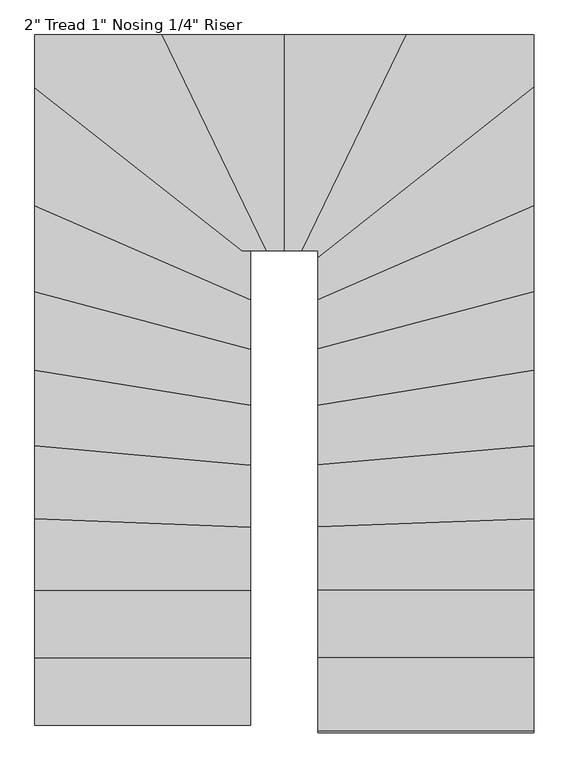
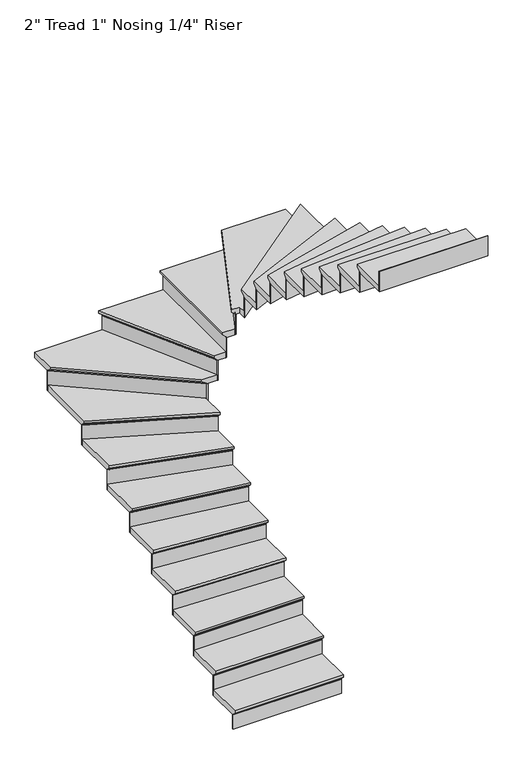
"""IFC4 building model written with IfcOpenShell, lengths in millimetres: stair flight geometry."""

from ifc_helpers import new_model, si_unit, origin, place, context, project, spatial, faceted_brep, source, transform, mapped, element, save


def stair_flight_464fb83d(model_context):
    return source(origin(), model_context, "Body", "Brep", [
        faceted_brep([(-5047.1987704, -4554.2130548, 33073.5214286), (-5047.1987704, -4554.2130548, 33092.5714286), (-5940.8822214, -4554.2130548, 33092.5714286), (-5940.8822214, -4554.2130548, 33073.5214286), (-5047.1987704, -4528.8130548, 33048.1214286), (-5940.8822214, -4528.8130548, 33048.1214286), (-5047.1987704, -4249.4130548, 33092.5714286), (-5940.8822214, -4249.4130548, 33092.5714286), (-5940.8822214, -4528.8130548, 33041.7714286), (-5940.8822214, -4249.4130548, 33041.7714286), (-5047.1987704, -4249.4130548, 33041.7714286), (-5047.1987704, -4528.8130548, 33041.7714286)], [[[0, 1, 2, 3]], [[4, 0, 3, 5]], [[2, 1, 6, 7]], [[8, 9, 10, 11]], [[2, 7, 9, 8, 5, 3]], [[8, 11, 4, 5]], [[6, 1, 0, 4, 11, 10]], [[7, 6, 10, 9]]]),
        faceted_brep([(-5047.1987704, -4528.8130548, 33041.7714286), (-5047.1987704, -4528.8130548, 32918.4), (-5047.1987704, -4522.4630548, 32918.4), (-5047.1987704, -4522.4630548, 33041.7714286), (-5940.8822214, -4528.8130548, 33041.7714286), (-5940.8822214, -4522.4630548, 33041.7714286), (-5940.8822214, -4522.4630548, 32918.4), (-5940.8822214, -4528.8130548, 32918.4)], [[[0, 1, 2, 3]], [[4, 5, 6, 7]], [[1, 0, 4, 7]], [[2, 1, 7, 6]], [[3, 2, 6, 5]], [[0, 3, 5, 4]]]),
        faceted_brep([(-5047.1987704, -4249.4130548, 33215.9428571), (-5047.1987704, -4249.4130548, 33041.7714286), (-5047.1987704, -4243.0630548, 33041.7714286), (-5047.1987704, -4243.0630548, 33215.9428571), (-5940.8822214, -4249.4130548, 33215.9428571), (-5940.8822214, -4243.0630548, 33215.9428571), (-5940.8822214, -4243.0630548, 33041.7714286), (-5940.8822214, -4249.4130548, 33041.7714286)], [[[0, 1, 2, 3]], [[4, 5, 6, 7]], [[1, 0, 4, 7]], [[2, 1, 7, 6]], [[3, 2, 6, 5]], [[0, 3, 5, 4]]]),
        faceted_brep([(-5940.8822214, -4274.8130548, 33266.7428571), (-5047.1987704, -4274.8130548, 33266.7428571), (-5047.1987704, -3970.0130548, 33266.7428571), (-5940.8822214, -3970.0130548, 33266.7428571), (-5940.8822214, -4249.4130548, 33215.9428571), (-5940.8822214, -3970.0130548, 33215.9428571), (-5047.1987704, -3970.0130548, 33215.9428571), (-5047.1987704, -4249.4130548, 33215.9428571), (-5940.8822214, -4249.4130548, 33222.2928571), (-5940.8822214, -4274.8130548, 33247.6928571), (-5047.1987704, -4249.4130548, 33222.2928571), (-5047.1987704, -4274.8130548, 33247.6928571)], [[[0, 1, 2, 3]], [[4, 5, 6, 7]], [[0, 3, 5, 4, 8, 9]], [[4, 7, 10, 8]], [[2, 1, 11, 10, 7, 6]], [[3, 2, 6, 5]], [[11, 1, 0, 9]], [[10, 11, 9, 8]]]),
        faceted_brep([(-5047.1987704, -3970.0130548, 33390.1142857), (-5047.1987704, -3970.0130548, 33215.9428571), (-5047.1987704, -3963.6630548, 33215.9428571), (-5047.1987704, -3963.6630548, 33390.1142857), (-5940.8822214, -3970.0130548, 33390.1142857), (-5940.8822214, -3963.6630548, 33390.1142857), (-5940.8822214, -3963.6630548, 33215.9428571), (-5940.8822214, -3970.0130548, 33215.9428571)], [[[0, 1, 2, 3]], [[4, 5, 6, 7]], [[1, 0, 4, 7]], [[2, 1, 7, 6]], [[3, 2, 6, 5]], [[0, 3, 5, 4]]]),
        faceted_brep([(-5940.8822214, -3995.4130548, 33440.9142857), (-5047.1987704, -3995.4130548, 33440.9142857), (-5047.1987704, -3707.9036879, 33440.9142857), (-5940.8822214, -3673.2843203, 33440.9142857), (-5940.8822214, -3970.0130548, 33390.1142857), (-5940.8822214, -3673.2843203, 33390.1142857), (-5047.1987704, -3707.9036879, 33390.1142857), (-5047.1987704, -3970.0130548, 33390.1142857), (-5940.8822214, -3970.0130548, 33396.4642857), (-5940.8822214, -3995.4130548, 33421.8642857), (-5047.1987704, -3970.0130548, 33396.4642857), (-5047.1987704, -3995.4130548, 33421.8642857)], [[[0, 1, 2, 3]], [[4, 5, 6, 7]], [[0, 3, 5, 4, 8, 9]], [[4, 7, 10, 8]], [[2, 1, 11, 10, 7, 6]], [[3, 2, 6, 5]], [[11, 1, 0, 9]], [[10, 11, 9, 8]]]),
        faceted_brep([(-5047.1987704, -3707.9036879, 33564.2857143), (-5047.1987704, -3707.9036879, 33390.1142857), (-5047.1987704, -3701.5489252, 33390.1142857), (-5047.1987704, -3701.5489252, 33564.2857143), (-5940.8822214, -3673.2843203, 33564.2857143), (-5940.8822214, -3666.9295576, 33564.2857143), (-5940.8822214, -3666.9295576, 33390.1142857), (-5940.8822214, -3673.2843203, 33390.1142857)], [[[0, 1, 2, 3]], [[4, 5, 6, 7]], [[1, 0, 4, 7]], [[2, 1, 7, 6]], [[3, 2, 6, 5]], [[0, 3, 5, 4]]]),
        faceted_brep([(-5940.8822214, -3698.703371, 33615.0857143), (-5047.1987704, -3733.3227386, 33615.0857143), (-5047.1987704, -3451.3234819, 33615.0857143), (-5940.8822214, -3370.89733, 33615.0857143), (-5940.8822214, -3673.2843203, 33564.2857143), (-5940.8822214, -3370.89733, 33564.2857143), (-5047.1987704, -3451.3234819, 33564.2857143), (-5047.1987704, -3707.9036879, 33564.2857143), (-5940.8822214, -3673.2843203, 33570.6357143), (-5940.8822214, -3698.703371, 33596.0357143), (-5047.1987704, -3707.9036879, 33570.6357143), (-5047.1987704, -3733.3227386, 33596.0357143)], [[[0, 1, 2, 3]], [[4, 5, 6, 7]], [[0, 3, 5, 4, 8, 9]], [[4, 7, 10, 8]], [[2, 1, 11, 10, 7, 6]], [[3, 2, 6, 5]], [[11, 1, 0, 9]], [[10, 11, 9, 8]]]),
        faceted_brep([(-5047.1987704, -3451.3234819, 33738.4571429), (-5047.1987704, -3451.3234819, 33564.2857143), (-5047.1987704, -3444.9478197, 33564.2857143), (-5047.1987704, -3444.9478197, 33738.4571429), (-5940.8822214, -3370.89733, 33738.4571429), (-5940.8822214, -3364.5216678, 33738.4571429), (-5940.8822214, -3364.5216678, 33564.2857143), (-5940.8822214, -3370.89733, 33564.2857143)], [[[0, 1, 2, 3]], [[4, 5, 6, 7]], [[1, 0, 4, 7]], [[2, 1, 7, 6]], [[3, 2, 6, 5]], [[0, 3, 5, 4]]]),
        faceted_brep([(-5940.8822214, -3396.3999789, 33789.2571429), (-5047.1987704, -3476.8261308, 33789.2571429), (-5047.1987704, -3203.4301079, 33789.2571429), (-5940.8822214, -3059.5417727, 33789.2571429), (-5940.8822214, -3370.89733, 33738.4571429), (-5940.8822214, -3059.5417727, 33738.4571429), (-5047.1987704, -3203.4301079, 33738.4571429), (-5047.1987704, -3451.3234819, 33738.4571429), (-5940.8822214, -3370.89733, 33744.8071429), (-5940.8822214, -3396.3999789, 33770.2071429), (-5047.1987704, -3451.3234819, 33744.8071429), (-5047.1987704, -3476.8261308, 33770.2071429)], [[[0, 1, 2, 3]], [[4, 5, 6, 7]], [[0, 3, 5, 4, 8, 9]], [[4, 7, 10, 8]], [[2, 1, 11, 10, 7, 6]], [[3, 2, 6, 5]], [[11, 1, 0, 9]], [[10, 11, 9, 8]]]),
        faceted_brep([(-5047.1987704, -3203.4301079, 33912.6285714), (-5047.1987704, -3203.4301079, 33738.4571429), (-5047.1987704, -3196.9983292, 33738.4571429), (-5047.1987704, -3196.9983292, 33912.6285714), (-5940.8822214, -3059.5417727, 33912.6285714), (-5940.8822214, -3053.109994, 33912.6285714), (-5940.8822214, -3053.109994, 33738.4571429), (-5940.8822214, -3059.5417727, 33738.4571429)], [[[0, 1, 2, 3]], [[4, 5, 6, 7]], [[1, 0, 4, 7]], [[2, 1, 7, 6]], [[3, 2, 6, 5]], [[0, 3, 5, 4]]]),
        faceted_brep([(-5940.8822214, -3085.2688872, 33963.4285714), (-5047.1987704, -3229.1572224, 33963.4285714), (-5047.1987704, -2970.3553609, 33963.4285714), (-5940.8822214, -2732.7052783, 33963.4285714), (-5940.8822214, -3059.5417727, 33912.6285714), (-5940.8822214, -2732.7052783, 33912.6285714), (-5047.1987704, -2970.3553609, 33912.6285714), (-5047.1987704, -3203.4301079, 33912.6285714), (-5940.8822214, -3059.5417727, 33918.9785714), (-5940.8822214, -3085.2688872, 33944.3785714), (-5047.1987704, -3203.4301079, 33918.9785714), (-5047.1987704, -3229.1572224, 33944.3785714)], [[[0, 1, 2, 3]], [[4, 5, 6, 7]], [[0, 3, 5, 4, 8, 9]], [[4, 7, 10, 8]], [[2, 1, 11, 10, 7, 6]], [[3, 2, 6, 5]], [[11, 1, 0, 9]], [[10, 11, 9, 8]]]),
        faceted_brep([(-5047.1987704, -2970.3553609, 34086.8), (-5047.1987704, -2970.3553609, 33912.6285714), (-5047.1987704, -2963.7846771, 33912.6285714), (-5047.1987704, -2963.7846771, 34086.8), (-5940.8822214, -2732.7052783, 34086.8), (-5940.8822214, -2726.1345945, 34086.8), (-5940.8822214, -2726.1345945, 33912.6285714), (-5940.8822214, -2732.7052783, 33912.6285714)], [[[0, 1, 2, 3]], [[4, 5, 6, 7]], [[1, 0, 4, 7]], [[2, 1, 7, 6]], [[3, 2, 6, 5]], [[0, 3, 5, 4]]]),
        faceted_brep([(-5940.8822214, -2758.9880136, 34137.6), (-5047.1987704, -2996.6380961, 34137.6), (-5047.1987704, -2765.8050203, 34137.6), (-5940.8822214, -2375.5896532, 34137.6), (-5940.8822214, -2732.7052783, 34086.8), (-5940.8822214, -2375.5896532, 34086.8), (-5047.1987704, -2765.8050203, 34086.8), (-5047.1987704, -2970.3553609, 34086.8), (-5940.8822214, -2732.7052783, 34093.15), (-5940.8822214, -2758.9880136, 34118.55), (-5047.1987704, -2970.3553609, 34093.15), (-5047.1987704, -2996.6380961, 34118.55)], [[[0, 1, 2, 3]], [[4, 5, 6, 7]], [[0, 3, 5, 4, 8, 9]], [[4, 7, 10, 8]], [[2, 1, 11, 10, 7, 6]], [[3, 2, 6, 5]], [[11, 1, 0, 9]], [[10, 11, 9, 8]]]),
        faceted_brep([(-5047.1987704, -2765.8050203, 34260.9714286), (-5047.1987704, -2765.8050203, 34086.8), (-5047.1987704, -2758.8760908, 34086.8), (-5047.1987704, -2758.8760908, 34260.9714286), (-5940.8822214, -2375.5896532, 34260.9714286), (-5940.8822214, -2368.6607237, 34260.9714286), (-5940.8822214, -2368.6607237, 34086.8), (-5940.8822214, -2375.5896532, 34086.8)], [[[0, 1, 2, 3]], [[4, 5, 6, 7]], [[1, 0, 4, 7]], [[2, 1, 7, 6]], [[3, 2, 6, 5]], [[0, 3, 5, 4]]]),
        faceted_brep([(-5940.8822214, -2403.3053713, 34311.7714286), (-5047.1987704, -2793.5207384, 34311.7714286), (-5047.1987704, -2590.8424524, 34311.7714286), (-5040.8038639, -2590.8424524, 34311.7714286), (-5940.8822214, -1882.1944717, 34311.7714286), (-5940.8822214, -2375.5896532, 34260.9714286), (-5940.8822214, -1882.1944717, 34260.9714286), (-5040.8038639, -2590.8424524, 34260.9714286), (-5047.1987704, -2590.8424524, 34260.9714286), (-5047.1987704, -2765.8050203, 34260.9714286), (-5940.8822214, -2375.5896532, 34267.3214286), (-5940.8822214, -2403.3053713, 34292.7214286), (-5047.1987704, -2765.8050203, 34267.3214286), (-5047.1987704, -2793.5207384, 34292.7214286)], [[[0, 1, 2, 3, 4]], [[5, 6, 7, 8, 9]], [[0, 4, 6, 5, 10, 11]], [[5, 9, 12, 10]], [[2, 1, 13, 12, 9, 8]], [[4, 3, 7, 6]], [[13, 1, 0, 11]], [[12, 13, 11, 10]], [[3, 2, 8, 7]]]),
        faceted_brep([(-5040.8038639, -2590.8424524, 34435.1428571), (-5040.8038639, -2590.8424524, 34260.9714286), (-5030.5387554, -2590.8424524, 34260.9714286), (-5030.5387554, -2590.8424524, 34435.1428571), (-5940.8822214, -1882.1944717, 34435.1428571), (-5940.8822214, -1874.1125661, 34435.1428571), (-5940.8822214, -1874.1125661, 34260.9714286), (-5940.8822214, -1882.1944717, 34260.9714286)], [[[0, 1, 2, 3]], [[4, 5, 6, 7]], [[1, 0, 4, 7]], [[2, 1, 7, 6]], [[3, 2, 6, 5]], [[0, 3, 5, 4]]]),
        faceted_brep([(-5384.6489457, -1697.1590014, 34485.9428571), (-5940.8822214, -1697.1590014, 34485.9428571), (-5940.8822214, -1914.5220945, 34485.9428571), (-5081.8642978, -2590.8424524, 34485.9428571), (-4952.3566185, -2590.8424524, 34485.9428571), (-5940.8822214, -1697.1590014, 34435.1428571), (-5384.6489457, -1697.1590014, 34435.1428571), (-4952.3566185, -2590.8424524, 34435.1428571), (-5040.8038639, -2590.8424524, 34435.1428571), (-5940.8822214, -1882.1944717, 34435.1428571), (-5940.8822214, -1882.1944717, 34441.4928571), (-5940.8822214, -1914.5220945, 34466.8928571), (-5040.8038639, -2590.8424524, 34441.4928571), (-5081.8642978, -2590.8424524, 34466.8928571)], [[[0, 1, 2, 3, 4]], [[5, 6, 7, 8, 9]], [[1, 0, 6, 5]], [[2, 1, 5, 9, 10, 11]], [[9, 8, 12, 10]], [[4, 3, 13, 12, 8, 7]], [[0, 4, 7, 6]], [[13, 3, 2, 11]], [[12, 13, 11, 10]]]),
        faceted_brep([(-4952.3566185, -2590.8424524, 34609.3142857), (-4952.3566185, -2590.8424524, 34435.1428571), (-4945.3027294, -2590.8424524, 34435.1428571), (-4945.3027294, -2590.8424524, 34609.3142857), (-5384.6489457, -1697.1590014, 34609.3142857), (-5377.5950566, -1697.1590014, 34609.3142857), (-5377.5950566, -1697.1590014, 34435.1428571), (-5384.6489457, -1697.1590014, 34435.1428571)], [[[0, 1, 2, 3]], [[4, 5, 6, 7]], [[1, 0, 4, 7]], [[2, 1, 7, 6]], [[3, 2, 6, 5]], [[0, 3, 5, 4]]]),
        faceted_brep([(-5412.8645022, -1697.1590014, 34660.1142857), (-4980.5721749, -2590.8424524, 34660.1142857), (-4882.0987704, -2590.8424524, 34660.1142857), (-4882.0987706, -1697.1590014, 34660.1142857), (-5384.6489457, -1697.1590014, 34609.3142857), (-4882.0987706, -1697.1590014, 34609.3142857), (-4882.0987704, -2590.8424524, 34609.3142857), (-4952.3566185, -2590.8424524, 34609.3142857), (-5384.6489457, -1697.1590014, 34615.6642857), (-5412.8645022, -1697.1590014, 34641.0642857), (-4952.3566185, -2590.8424524, 34615.6642857), (-4980.5721749, -2590.8424524, 34641.0642857)], [[[0, 1, 2, 3]], [[4, 5, 6, 7]], [[0, 3, 5, 4, 8, 9]], [[4, 7, 10, 8]], [[3, 2, 6, 5]], [[11, 1, 0, 9]], [[10, 11, 9, 8]], [[2, 1, 11, 10, 7, 6]]]),
        faceted_brep([(-4882.0987704, -2590.8424524, 34783.4857143), (-4882.0987704, -2590.8424524, 34609.3142857), (-4875.7487704, -2590.8424524, 34609.3142857), (-4875.7487704, -2590.8424524, 34783.4857143), (-4882.0987706, -1697.1590014, 34783.4857143), (-4875.7487706, -1697.1590014, 34783.4857143), (-4875.7487706, -1697.1590014, 34609.3142857), (-4882.0987706, -1697.1590014, 34609.3142857)], [[[0, 1, 2, 3]], [[4, 5, 6, 7]], [[1, 0, 4, 7]], [[2, 1, 7, 6]], [[3, 2, 6, 5]], [[0, 3, 5, 4]]]),
        faceted_brep([(-4907.4987706, -1697.1590014, 34834.2857143), (-4907.4987704, -2590.8424524, 34834.2857143), (-4806.2098095, -2590.8424524, 34834.2857143), (-4373.9174828, -1697.1590014, 34834.2857143), (-4882.0987706, -1697.1590014, 34783.4857143), (-4373.9174828, -1697.1590014, 34783.4857143), (-4806.2098095, -2590.8424524, 34783.4857143), (-4882.0987704, -2590.8424524, 34783.4857143), (-4882.0987706, -1697.1590014, 34789.8357143), (-4907.4987706, -1697.1590014, 34815.2357143), (-4882.0987704, -2590.8424524, 34789.8357143), (-4907.4987704, -2590.8424524, 34815.2357143)], [[[0, 1, 2, 3]], [[4, 5, 6, 7]], [[0, 3, 5, 4, 8, 9]], [[4, 7, 10, 8]], [[2, 1, 11, 10, 7, 6]], [[3, 2, 6, 5]], [[11, 1, 0, 9]], [[10, 11, 9, 8]]]),
        faceted_brep([(-4806.2098095, -2590.8424524, 34957.6571429), (-4806.2098095, -2590.8424524, 34783.4857143), (-4799.1559204, -2590.8424524, 34783.4857143), (-4799.1559204, -2590.8424524, 34957.6571429), (-4373.9174828, -1697.1590014, 34957.6571429), (-4366.8635937, -1697.1590014, 34957.6571429), (-4366.8635937, -1697.1590014, 34783.4857143), (-4373.9174828, -1697.1590014, 34783.4857143)], [[[0, 1, 2, 3]], [[4, 5, 6, 7]], [[1, 0, 4, 7]], [[2, 1, 7, 6]], [[3, 2, 6, 5]], [[0, 3, 5, 4]]]),
        faceted_brep([(-3874.1153195, -1946.8497166, 35008.4571429), (-3874.1153195, -1697.1590014, 35008.4571429), (-4402.1330392, -1697.1590014, 35008.4571429), (-4834.4253659, -2590.8424524, 35008.4571429), (-4767.7987704, -2590.8424524, 35008.4571429), (-4767.7987704, -2650.4628721, 35008.4571429), (-3874.1153195, -1697.1590014, 34957.6571429), (-3874.1153195, -1946.8497166, 34957.6571429), (-4767.7987704, -2650.4628721, 34957.6571429), (-4767.7987704, -2590.8424524, 34957.6571429), (-4806.2098095, -2590.8424524, 34957.6571429), (-4373.9174828, -1697.1590014, 34957.6571429), (-4806.2098095, -2590.8424524, 34964.0071429), (-4373.9174828, -1697.1590014, 34964.0071429), (-4834.4253659, -2590.8424524, 34989.4071429), (-4402.1330392, -1697.1590014, 34989.4071429)], [[[0, 1, 2, 3, 4, 5]], [[6, 7, 8, 9, 10, 11]], [[1, 0, 7, 6]], [[11, 10, 12, 13]], [[4, 3, 14, 12, 10, 9]], [[5, 4, 9, 8]], [[0, 5, 8, 7]], [[14, 3, 2, 15]], [[12, 14, 15, 13]], [[2, 1, 6, 11, 13, 15]]]),
        faceted_brep([(-4767.7987704, -2650.4628721, 35131.8285714), (-4767.7987704, -2650.4628721, 34957.6571429), (-4767.7987704, -2658.5447778, 34957.6571429), (-4767.7987704, -2658.5447778, 35131.8285714), (-3874.1153195, -1946.8497166, 35131.8285714), (-3874.1153195, -1954.9316222, 35131.8285714), (-3874.1153195, -1954.9316222, 34957.6571429), (-3874.1153195, -1946.8497166, 34957.6571429)], [[[0, 1, 2, 3]], [[4, 5, 6, 7]], [[1, 0, 4, 7]], [[2, 1, 7, 6]], [[3, 2, 6, 5]], [[0, 3, 5, 4]]]),
        faceted_brep([(-3874.1153195, -1914.5220938, 35182.6285714), (-4767.7987704, -2618.1352494, 35182.6285714), (-4767.7987704, -2821.2364563, 35182.6285714), (-3874.1153195, -2431.0210889, 35182.6285714), (-3874.1153195, -1946.8497166, 35131.8285714), (-3874.1153195, -2431.0210889, 35131.8285714), (-4767.7987704, -2821.2364563, 35131.8285714), (-4767.7987704, -2650.4628721, 35131.8285714), (-3874.1153195, -1946.8497166, 35138.1785714), (-3874.1153195, -1914.5220938, 35163.5785714), (-4767.7987704, -2650.4628721, 35138.1785714), (-4767.7987704, -2618.1352494, 35163.5785714)], [[[0, 1, 2, 3]], [[4, 5, 6, 7]], [[0, 3, 5, 4, 8, 9]], [[4, 7, 10, 8]], [[2, 1, 11, 10, 7, 6]], [[3, 2, 6, 5]], [[11, 1, 0, 9]], [[10, 11, 9, 8]]]),
        faceted_brep([(-4767.7987704, -2821.2364563, 35306.0), (-4767.7987704, -2821.2364563, 35131.8285714), (-4767.7987704, -2828.1653858, 35131.8285714), (-4767.7987704, -2828.1653858, 35306.0), (-3874.1153195, -2431.0210889, 35306.0), (-3874.1153195, -2437.9500185, 35306.0), (-3874.1153195, -2437.9500185, 35131.8285714), (-3874.1153195, -2431.0210889, 35131.8285714)], [[[0, 1, 2, 3]], [[4, 5, 6, 7]], [[1, 0, 4, 7]], [[2, 1, 7, 6]], [[3, 2, 6, 5]], [[0, 3, 5, 4]]]),
        faceted_brep([(-3874.1153195, -2403.3053709, 35356.8), (-4767.7987704, -2793.5207382, 35356.8), (-4767.7987704, -3022.9208311, 35356.8), (-3874.1153195, -2785.2707484, 35356.8), (-3874.1153195, -2431.0210889, 35306.0), (-3874.1153195, -2785.2707484, 35306.0), (-4767.7987704, -3022.9208311, 35306.0), (-4767.7987704, -2821.2364563, 35306.0), (-3874.1153195, -2431.0210889, 35312.35), (-3874.1153195, -2403.3053709, 35337.75), (-4767.7987704, -2821.2364563, 35312.35), (-4767.7987704, -2793.5207382, 35337.75)], [[[0, 1, 2, 3]], [[4, 5, 6, 7]], [[0, 3, 5, 4, 8, 9]], [[4, 7, 10, 8]], [[2, 1, 11, 10, 7, 6]], [[3, 2, 6, 5]], [[11, 1, 0, 9]], [[10, 11, 9, 8]]]),
        faceted_brep([(-4767.7987704, -3022.9208311, 35480.1714286), (-4767.7987704, -3022.9208311, 35306.0), (-4767.7987704, -3029.4915149, 35306.0), (-4767.7987704, -3029.4915149, 35480.1714286), (-3874.1153195, -2785.2707484, 35480.1714286), (-3874.1153195, -2791.8414322, 35480.1714286), (-3874.1153195, -2791.8414322, 35306.0), (-3874.1153195, -2785.2707484, 35306.0)], [[[0, 1, 2, 3]], [[4, 5, 6, 7]], [[1, 0, 4, 7]], [[2, 1, 7, 6]], [[3, 2, 6, 5]], [[0, 3, 5, 4]]]),
        faceted_brep([(-3874.1153195, -2758.9880132, 35530.9714286), (-4767.7987704, -2996.6380959, 35530.9714286), (-4767.7987704, -3254.8843368, 35530.9714286), (-3874.1153195, -3110.9960015, 35530.9714286), (-3874.1153195, -2785.2707484, 35480.1714286), (-3874.1153195, -3110.9960015, 35480.1714286), (-4767.7987704, -3254.8843368, 35480.1714286), (-4767.7987704, -3022.9208311, 35480.1714286), (-3874.1153195, -2785.2707484, 35486.5214286), (-3874.1153195, -2758.9880132, 35511.9214286), (-4767.7987704, -3022.9208311, 35486.5214286), (-4767.7987704, -2996.6380959, 35511.9214286)], [[[0, 1, 2, 3]], [[4, 5, 6, 7]], [[0, 3, 5, 4, 8, 9]], [[4, 7, 10, 8]], [[2, 1, 11, 10, 7, 6]], [[3, 2, 6, 5]], [[11, 1, 0, 9]], [[10, 11, 9, 8]]]),
        faceted_brep([(-4767.7987704, -3254.8843368, 35654.3428571), (-4767.7987704, -3254.8843368, 35480.1714286), (-4767.7987704, -3261.3161154, 35480.1714286), (-4767.7987704, -3261.3161154, 35654.3428571), (-3874.1153195, -3110.9960015, 35654.3428571), (-3874.1153195, -3117.4277801, 35654.3428571), (-3874.1153195, -3117.4277801, 35480.1714286), (-3874.1153195, -3110.9960015, 35480.1714286)], [[[0, 1, 2, 3]], [[4, 5, 6, 7]], [[1, 0, 4, 7]], [[2, 1, 7, 6]], [[3, 2, 6, 5]], [[0, 3, 5, 4]]]),
        faceted_brep([(-3874.1153195, -3085.2688869, 35705.1428571), (-4767.7987704, -3229.1572222, 35705.1428571), (-4767.7987704, -3502.3287795, 35705.1428571), (-3874.1153195, -3421.9026274, 35705.1428571), (-3874.1153195, -3110.9960015, 35654.3428571), (-3874.1153195, -3421.9026274, 35654.3428571), (-4767.7987704, -3502.3287795, 35654.3428571), (-4767.7987704, -3254.8843368, 35654.3428571), (-3874.1153195, -3110.9960015, 35660.6928571), (-3874.1153195, -3085.2688869, 35686.0928571), (-4767.7987704, -3254.8843368, 35660.6928571), (-4767.7987704, -3229.1572222, 35686.0928571)], [[[0, 1, 2, 3]], [[4, 5, 6, 7]], [[0, 3, 5, 4, 8, 9]], [[4, 7, 10, 8]], [[2, 1, 11, 10, 7, 6]], [[3, 2, 6, 5]], [[11, 1, 0, 9]], [[10, 11, 9, 8]]]),
        faceted_brep([(-4767.7987704, -3502.3287795, 35828.5142857), (-4767.7987704, -3502.3287795, 35654.3428571), (-4767.7987704, -3508.7044417, 35654.3428571), (-4767.7987704, -3508.7044417, 35828.5142857), (-3874.1153195, -3421.9026274, 35828.5142857), (-3874.1153195, -3428.2782897, 35828.5142857), (-3874.1153195, -3428.2782897, 35654.3428571), (-3874.1153195, -3421.9026274, 35654.3428571)], [[[0, 1, 2, 3]], [[4, 5, 6, 7]], [[1, 0, 4, 7]], [[2, 1, 7, 6]], [[3, 2, 6, 5]], [[0, 3, 5, 4]]]),
        faceted_brep([(-3874.1153195, -3396.3999786, 35879.3142857), (-4767.7987704, -3476.8261306, 35879.3142857), (-4767.7987704, -3758.7417891, 35879.3142857), (-3874.1153195, -3724.1224215, 35879.3142857), (-3874.1153195, -3421.9026274, 35828.5142857), (-3874.1153195, -3724.1224215, 35828.5142857), (-4767.7987704, -3758.7417891, 35828.5142857), (-4767.7987704, -3502.3287795, 35828.5142857), (-3874.1153195, -3421.9026274, 35834.8642857), (-3874.1153195, -3396.3999786, 35860.2642857), (-4767.7987704, -3502.3287795, 35834.8642857), (-4767.7987704, -3476.8261306, 35860.2642857)], [[[0, 1, 2, 3]], [[4, 5, 6, 7]], [[0, 3, 5, 4, 8, 9]], [[4, 7, 10, 8]], [[2, 1, 11, 10, 7, 6]], [[3, 2, 6, 5]], [[11, 1, 0, 9]], [[10, 11, 9, 8]]]),
        faceted_brep([(-4767.7987704, -3758.7417891, 36002.6857143), (-4767.7987704, -3758.7417891, 35828.5142857), (-4767.7987704, -3765.0965518, 35828.5142857), (-4767.7987704, -3765.0965518, 36002.6857143), (-3874.1153195, -3724.1224215, 36002.6857143), (-3874.1153195, -3730.4771842, 36002.6857143), (-3874.1153195, -3730.4771842, 35828.5142857), (-3874.1153195, -3724.1224215, 35828.5142857)], [[[0, 1, 2, 3]], [[4, 5, 6, 7]], [[1, 0, 4, 7]], [[2, 1, 7, 6]], [[3, 2, 6, 5]], [[0, 3, 5, 4]]]),
        faceted_brep([(-3874.1153195, -3698.7033708, 36053.4857143), (-4767.7987704, -3733.3227384, 36053.4857143), (-4767.7987704, -4020.8130546, 36053.4857143), (-3874.1153195, -4020.8130546, 36053.4857143), (-3874.1153195, -3724.1224215, 36002.6857143), (-3874.1153195, -4020.8130546, 36002.6857143), (-4767.7987704, -4020.8130546, 36002.6857143), (-4767.7987704, -3758.7417891, 36002.6857143), (-3874.1153195, -3724.1224215, 36009.0357143), (-3874.1153195, -3698.7033708, 36034.4357143), (-4767.7987704, -3758.7417891, 36009.0357143), (-4767.7987704, -3733.3227384, 36034.4357143)], [[[0, 1, 2, 3]], [[4, 5, 6, 7]], [[0, 3, 5, 4, 8, 9]], [[4, 7, 10, 8]], [[2, 1, 11, 10, 7, 6]], [[3, 2, 6, 5]], [[11, 1, 0, 9]], [[10, 11, 9, 8]]]),
        faceted_brep([(-4767.7987704, -4020.8130546, 36176.8571429), (-4767.7987704, -4020.8130546, 36002.6857143), (-4767.7987704, -4027.1630546, 36002.6857143), (-4767.7987704, -4027.1630546, 36176.8571429), (-3874.1153195, -4020.8130546, 36176.8571429), (-3874.1153195, -4027.1630546, 36176.8571429), (-3874.1153195, -4027.1630546, 36002.6857143), (-3874.1153195, -4020.8130546, 36002.6857143)], [[[0, 1, 2, 3]], [[4, 5, 6, 7]], [[1, 0, 4, 7]], [[2, 1, 7, 6]], [[3, 2, 6, 5]], [[0, 3, 5, 4]]]),
        faceted_brep([(-3874.1153195, -3995.4130546, 36227.6571429), (-4767.7987704, -3995.4130546, 36227.6571429), (-4767.7987704, -4300.2130546, 36227.6571429), (-3874.1153195, -4300.2130546, 36227.6571429), (-3874.1153195, -4020.8130546, 36176.8571429), (-3874.1153195, -4300.2130546, 36176.8571429), (-4767.7987704, -4300.2130546, 36176.8571429), (-4767.7987704, -4020.8130546, 36176.8571429), (-3874.1153195, -4020.8130546, 36183.2071429), (-3874.1153195, -3995.4130546, 36208.6071429), (-4767.7987704, -4020.8130546, 36183.2071429), (-4767.7987704, -3995.4130546, 36208.6071429)], [[[0, 1, 2, 3]], [[4, 5, 6, 7]], [[0, 3, 5, 4, 8, 9]], [[4, 7, 10, 8]], [[2, 1, 11, 10, 7, 6]], [[3, 2, 6, 5]], [[11, 1, 0, 9]], [[10, 11, 9, 8]]]),
        faceted_brep([(-4767.7987704, -4300.2130546, 36351.0285714), (-4767.7987704, -4300.2130546, 36176.8571429), (-4767.7987704, -4306.5630546, 36176.8571429), (-4767.7987704, -4306.5630546, 36351.0285714), (-3874.1153195, -4300.2130546, 36351.0285714), (-3874.1153195, -4306.5630546, 36351.0285714), (-3874.1153195, -4306.5630546, 36176.8571429), (-3874.1153195, -4300.2130546, 36176.8571429)], [[[0, 1, 2, 3]], [[4, 5, 6, 7]], [[1, 0, 4, 7]], [[2, 1, 7, 6]], [[3, 2, 6, 5]], [[0, 3, 5, 4]]]),
        faceted_brep([(-4767.7987704, -4579.6130546, 36525.2), (-4767.7987704, -4579.6130546, 36351.0285714), (-4767.7987704, -4585.9630546, 36351.0285714), (-4767.7987704, -4585.9630546, 36525.2), (-3874.1153195, -4579.6130546, 36525.2), (-3874.1153195, -4585.9630546, 36525.2), (-3874.1153195, -4585.9630546, 36351.0285714), (-3874.1153195, -4579.6130546, 36351.0285714)], [[[0, 1, 2, 3]], [[4, 5, 6, 7]], [[1, 0, 4, 7]], [[2, 1, 7, 6]], [[3, 2, 6, 5]], [[0, 3, 5, 4]]]),
        faceted_brep([(-3874.1153195, -4274.8130546, 36401.8285714), (-4767.7987704, -4274.8130546, 36401.8285714), (-4767.7987704, -4579.6130546, 36401.8285714), (-3874.1153195, -4579.6130546, 36401.8285714), (-3874.1153195, -4300.2130546, 36351.0285714), (-3874.1153195, -4579.6130546, 36351.0285714), (-4767.7987704, -4579.6130546, 36351.0285714), (-4767.7987704, -4300.2130546, 36351.0285714), (-3874.1153195, -4300.2130546, 36357.3785714), (-3874.1153195, -4274.8130546, 36382.7785714), (-4767.7987704, -4300.2130546, 36357.3785714), (-4767.7987704, -4274.8130546, 36382.7785714)], [[[0, 1, 2, 3]], [[4, 5, 6, 7]], [[0, 3, 5, 4, 8, 9]], [[4, 7, 10, 8]], [[2, 1, 11, 10, 7, 6]], [[3, 2, 6, 5]], [[11, 1, 0, 9]], [[10, 11, 9, 8]]]),
    ])


if __name__ == "__main__":
    model = new_model("IFC4")
    model_context = context("Model", 3, world=origin())
    ifc_project = project(units=[si_unit("LENGTHUNIT", "METRE", prefix="MILLI")], contexts=[model_context])
    site = spatial("IfcSite", under=ifc_project)
    building = spatial("IfcBuilding", under=site)
    placement = place(None, origin())
    stair_flight_shape = stair_flight_464fb83d(model_context)
    element("IfcStairFlight", 1, ObjectType="2\" Tread 1\" Nosing 1/4\" Riser", at=placement, inside=building, context=model_context, shape_type="MappedRepresentation", body=[
        mapped(stair_flight_shape, transform((0.0, 0.0, 0.0), x_axis=(1.0, 0.0, 0.0), y_axis=(0.0, 1.0, 0.0), z_axis=(0.0, 0.0, 1.0))),
    ])
    save(model, "model.ifc")

# Revit data of these elements
# Element 1 (IfcStairFlight, "2\" Tread 1\" Nosing 1/4\" Riser")
#   Materials on its faces: "Tile, Porcelain, 4in"
# Materials
#   "Tile, Porcelain, 4in": class "Generic", colour RGB 89 87 158, transparency 0, Description = "Porcelain tile, 4\", white", Cost = 0
